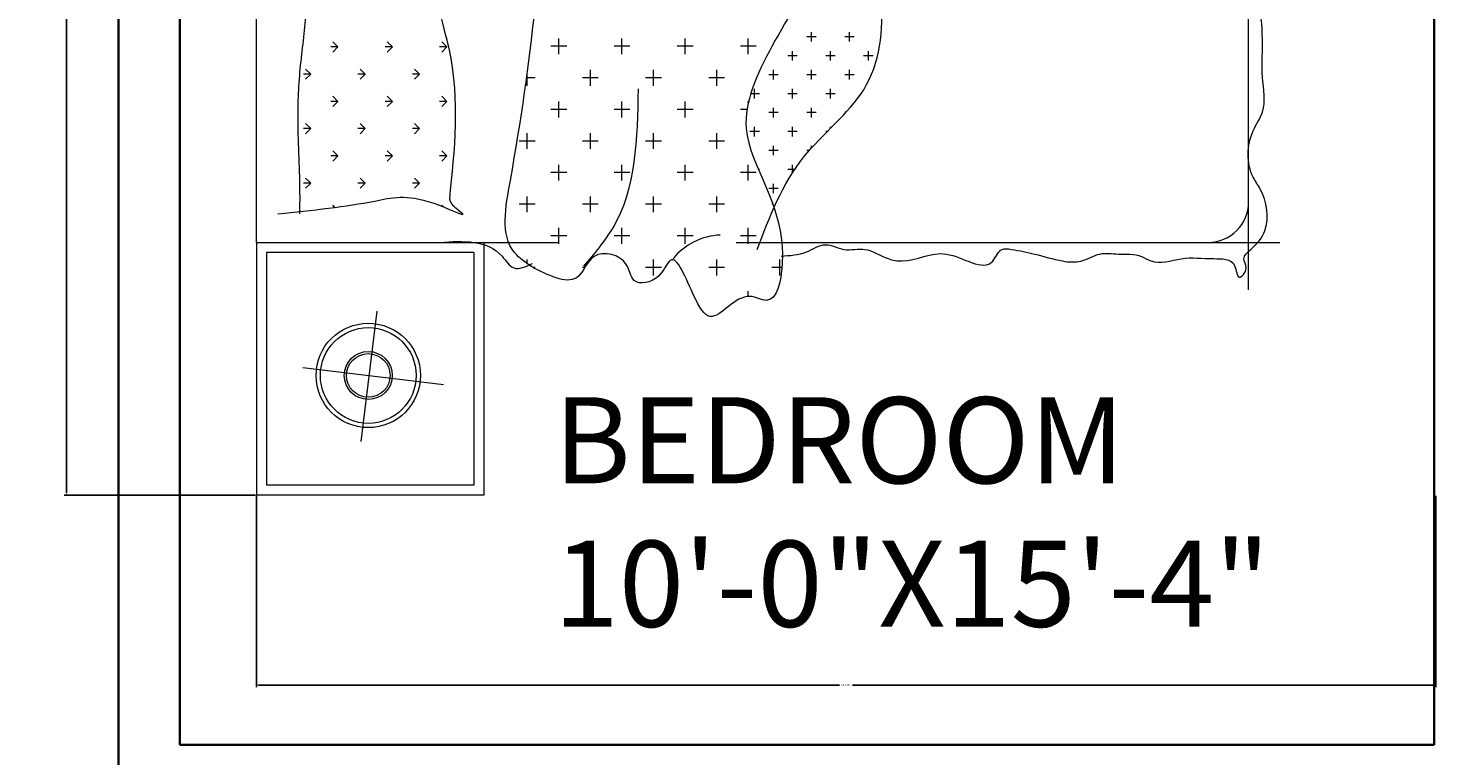
# Model space of a CAD drawing. Units: inches. Extents: x 3731 to 4318, y 1310 to 2388.
# Tile 3 of 57: x 3828 to 3944, y 1393 to 1452. Entities that reach past the tile are written whole.
import ezdxf

# ---------------------------------------------------------------- set-up
doc = ezdxf.new("R2010")
doc.units = ezdxf.units.IN
for name, color, linetype, lineweight in [('A-ANNO-DIMS', 2, 'Continuous', 18), ('A-AREA-IDEN', 7, 'Continuous', 18), ('A-FURN', 8, 'Continuous', 13), ('A-WALL', 7, 'Continuous', 35)]:
    doc.layers.add(name, color=color, linetype=linetype, lineweight=lineweight)
doc.styles.get("Standard").update_dxf_attribs({"font": 'arial.ttf'})
doc.dimstyles.get("Standard").update_dxf_attribs({"dimtxt": 0.18, "dimasz": 0.18, "dimexe": 0.18, "dimexo": 0.0625, "dimgap": 0.09, "dimtad": 0, "dimtih": 1, "dimtoh": 1, "dimdec": 4, "dimzin": 0, "dimdsep": 46, "dimtxsty": 'Standard', "dimcen": 0.09, "dimadec": 0, "dimazin": 0, "dimtfac": 1, "dimtdec": 4, "dimtofl": 0, "dimtmove": 0, "dimatfit": 3, "dimfxl": 1, "dimtolj": 1, "dimtzin": 0, "dimarcsym": 0})

# ---------------------------------------------------------------- blocks, each defined once
blk = doc.blocks.new('A$C200C7901')
for p, q in [((0, 1.8834), (0, 2.3334)), ((0.5, 2.3334), (0, 2.3334)), ((0.5, 2.3334), (0.5, 1.7369)), ((0.5, 2.3334), (0.5, 1.7369)), ((0.5, 2.3334), (2, 2.3334)), ((0.5701, 1.9635), (0.5733, 1.9666)), ((0.5701, 1.9635), (0.5733, 1.9666)), ((0.5, 1.8834), (0, 1.8834)), ((0.4504, 1.782), (0.4504, 1.7863)), ((0.4504, 1.782), (0.4504, 1.7863)), ((0.458, 1.7977), (0.466, 1.7977)), ((0.458, 1.7977), (0.466, 1.7977)), ((0.4504, 1.6834), (0.4504, 1.6883)), ((0.4504, 1.6834), (0.4504, 1.6883)), ((0.4656, 1.6727), (0.466, 1.6727)), ((0.4656, 1.6727), (0.466, 1.6727)), ((0.5597, 1.6727), (0.591, 1.6727)), ((0.5597, 1.6727), (0.591, 1.6727)), ((0.4504, 1.532), (0.4504, 1.5633)), ((0.4347, 1.5477), (0.466, 1.5477)), ((0.6847, 1.5477), (0.716, 1.5477)), ((0.4347, 1.4227), (0.466, 1.4227)), ((0.5, 1.3845), (0.5, 0.3086)), ((0.3931, 1.3602), (0.4035, 1.3602)), ((0.3931, 1.3602), (0.4035, 1.3602)), ((0.4972, 1.3602), (0.5285, 1.3602)), ((0.4972, 1.3602), (0.5285, 1.3602)), ((0.4347, 1.2977), (0.466, 1.2977)), ((0.4347, 1.2977), (0.466, 1.2977)), ((0.4504, 1.2936), (0.4504, 1.3133)), ((0.4504, 1.2936), (0.4504, 1.3133)), ((0.4061, 0.3703), (2.0386, 0.3703))]:
    blk.add_line(p, q)
at = {"linetype": 'ByBlock'}
for p, q in [((0.02, 1.9034), (0.02, 2.3134)), ((0.48, 2.3134), (0.02, 2.3134)), ((0.48, 1.9034), (0.48, 2.3134)), ((0.2524, 2.2412), (0.2186, 1.9635)), ((0.6171, 2.2259), (0.607, 2.236)), ((0.6171, 2.2259), (0.607, 2.236)), ((0.6171, 2.2259), (0.6171, 2.2402)), ((0.6171, 2.2259), (0.6171, 2.2402)), ((0.6171, 2.2259), (0.6272, 2.236)), ((0.6171, 2.2259), (0.6272, 2.236)), ((0.7249, 2.2259), (0.7148, 2.236)), ((0.7249, 2.2259), (0.7148, 2.236)), ((0.7249, 2.2259), (0.7249, 2.2402)), ((0.7249, 2.2259), (0.7249, 2.2402)), ((0.7249, 2.2259), (0.735, 2.236)), ((0.7249, 2.2259), (0.735, 2.236)), ((0.8326, 2.2259), (0.8225, 2.236)), ((0.8326, 2.2259), (0.8225, 2.236)), ((0.8326, 2.2259), (0.8326, 2.2402)), ((0.8326, 2.2259), (0.8326, 2.2402)), ((0.8326, 2.2259), (0.8427, 2.236)), ((0.8326, 2.2259), (0.8427, 2.236)), ((0.5692, 2.178), (0.5733, 2.1822)), ((0.5692, 2.178), (0.5733, 2.1822)), ((0.671, 2.1721), (0.6609, 2.1822)), ((0.671, 2.1721), (0.6609, 2.1822)), ((0.671, 2.172), (0.671, 2.1863)), ((0.671, 2.172), (0.671, 2.1863)), ((0.671, 2.1721), (0.6811, 2.1822)), ((0.671, 2.1721), (0.6811, 2.1822)), ((0.7787, 2.1721), (0.7686, 2.1822)), ((0.7787, 2.1721), (0.7686, 2.1822)), ((0.7787, 2.172), (0.7787, 2.1863)), ((0.7787, 2.172), (0.7787, 2.1863)), ((0.7787, 2.1721), (0.7889, 2.1822)), ((0.7787, 2.1721), (0.7889, 2.1822)), ((0.8865, 2.1721), (0.8764, 2.1822)), ((0.8865, 2.1721), (0.8764, 2.1822)), ((0.8865, 2.172), (0.8865, 2.1863)), ((0.8865, 2.172), (0.8865, 2.1863)), ((0.8865, 2.1721), (0.8966, 2.1822)), ((0.8865, 2.1721), (0.8966, 2.1822)), ((0.3641, 2.0951), (0.1061, 2.1268)), ((0.6171, 2.1182), (0.607, 2.1283)), ((0.6171, 2.1182), (0.607, 2.1283)), ((0.6171, 2.1182), (0.6171, 2.1325)), ((0.6171, 2.1182), (0.6171, 2.1325)), ((0.6171, 2.1182), (0.6272, 2.1283)), ((0.6171, 2.1182), (0.6272, 2.1283)), ((0.7249, 2.1182), (0.7148, 2.1283)), ((0.7249, 2.1182), (0.7148, 2.1283)), ((0.7249, 2.1182), (0.7249, 2.1325)), ((0.7249, 2.1182), (0.7249, 2.1325)), ((0.7249, 2.1182), (0.735, 2.1283)), ((0.7249, 2.1182), (0.735, 2.1283)), ((0.8326, 2.1182), (0.8225, 2.1283)), ((0.8326, 2.1182), (0.8225, 2.1283)), ((0.8326, 2.1182), (0.8326, 2.1325)), ((0.8326, 2.1182), (0.8326, 2.1325)), ((0.8326, 2.1182), (0.8427, 2.1283)), ((0.8326, 2.1182), (0.8427, 2.1283)), ((0.671, 2.0643), (0.6609, 2.0744)), ((0.671, 2.0643), (0.6609, 2.0744)), ((0.671, 2.0643), (0.671, 2.0786)), ((0.671, 2.0643), (0.671, 2.0786)), ((0.671, 2.0643), (0.6811, 2.0744)), ((0.671, 2.0643), (0.6811, 2.0744)), ((0.7787, 2.0643), (0.7686, 2.0744)), ((0.7787, 2.0643), (0.7686, 2.0744)), ((0.7787, 2.0643), (0.7787, 2.0786)), ((0.7787, 2.0643), (0.7787, 2.0786)), ((0.7787, 2.0643), (0.7889, 2.0744)), ((0.7787, 2.0643), (0.7889, 2.0744)), ((0.8865, 2.0643), (0.8764, 2.0744)), ((0.8865, 2.0643), (0.8764, 2.0744)), ((0.8865, 2.0643), (0.8865, 2.0786)), ((0.8865, 2.0643), (0.8865, 2.0786)), ((0.8865, 2.0643), (0.8966, 2.0744)), ((0.8865, 2.0643), (0.8966, 2.0744)), ((0.6171, 2.0104), (0.607, 2.0205)), ((0.6171, 2.0104), (0.607, 2.0205)), ((0.6171, 2.0104), (0.6171, 2.0247)), ((0.6171, 2.0104), (0.6171, 2.0247)), ((0.6171, 2.0104), (0.6272, 2.0205)), ((0.6171, 2.0104), (0.6272, 2.0205)), ((0.7249, 2.0104), (0.7148, 2.0205)), ((0.7249, 2.0104), (0.7148, 2.0205)), ((0.7249, 2.0104), (0.7249, 2.0247)), ((0.7249, 2.0104), (0.7249, 2.0247)), ((0.7249, 2.0104), (0.735, 2.0205)), ((0.7249, 2.0104), (0.735, 2.0205)), ((0.8326, 2.0104), (0.8225, 2.0205)), ((0.8326, 2.0104), (0.8225, 2.0205)), ((0.8326, 2.0104), (0.8326, 2.0247)), ((0.8326, 2.0104), (0.8326, 2.0247)), ((0.8326, 2.0104), (0.8427, 2.0205)), ((0.8326, 2.0104), (0.8427, 2.0205)), ((0.671, 1.9565), (0.6609, 1.9666)), ((0.671, 1.9565), (0.6609, 1.9666)), ((0.671, 1.9565), (0.671, 1.9708)), ((0.671, 1.9565), (0.671, 1.9708)), ((0.671, 1.9565), (0.6811, 1.9666)), ((0.671, 1.9565), (0.6811, 1.9666)), ((0.7787, 1.9565), (0.7686, 1.9666)), ((0.7787, 1.9565), (0.7686, 1.9666)), ((0.7787, 1.9565), (0.7787, 1.9708)), ((0.7787, 1.9565), (0.7787, 1.9708)), ((0.7787, 1.9565), (0.7889, 1.9666)), ((0.7787, 1.9565), (0.7889, 1.9666)), ((0.8865, 1.9565), (0.8764, 1.9666)), ((0.8865, 1.9565), (0.8764, 1.9666)), ((0.8865, 1.9565), (0.8865, 1.9708)), ((0.8865, 1.9565), (0.8865, 1.9708)), ((0.8865, 1.9565), (0.8966, 1.9666)), ((0.8865, 1.9565), (0.8966, 1.9666)), ((0.48, 1.9034), (0.02, 1.9034)), ((0.5754, 1.782), (0.5754, 1.8133)), ((0.5754, 1.782), (0.5754, 1.8133)), ((0.7004, 1.782), (0.7004, 1.8133)), ((0.7004, 1.782), (0.7004, 1.8133)), ((0.5597, 1.7977), (0.591, 1.7977)), ((0.5597, 1.7977), (0.591, 1.7977)), ((0.6847, 1.7977), (0.716, 1.7977)), ((0.6847, 1.7977), (0.716, 1.7977)), ((0.8097, 1.7977), (0.8331, 1.7977)), ((0.8097, 1.7977), (0.8331, 1.7977)), ((0.8254, 1.782), (0.8254, 1.7987)), ((0.8254, 1.782), (0.8254, 1.7987)), ((0.5129, 1.7195), (0.5129, 1.7508)), ((0.5129, 1.7195), (0.5129, 1.7508)), ((0.6379, 1.7195), (0.6379, 1.7508)), ((0.6379, 1.7195), (0.6379, 1.7508)), ((0.7629, 1.7195), (0.7629, 1.7508)), ((0.7629, 1.7195), (0.7629, 1.7508)), ((0.8879, 1.7195), (0.8879, 1.7508)), ((0.8879, 1.7195), (0.8879, 1.7508)), ((0.4972, 1.7352), (0.5285, 1.7352)), ((0.4972, 1.7352), (0.5285, 1.7352)), ((0.6222, 1.7352), (0.6535, 1.7352)), ((0.6222, 1.7352), (0.6535, 1.7352)), ((0.7472, 1.7352), (0.7785, 1.7352)), ((0.7472, 1.7352), (0.7785, 1.7352)), ((0.8722, 1.7352), (0.9035, 1.7352)), ((0.8722, 1.7352), (0.9035, 1.7352)), ((0.5754, 1.657), (0.5754, 1.6883)), ((0.5754, 1.657), (0.5754, 1.6883)), ((0.6847, 1.6727), (0.716, 1.6727)), ((0.6847, 1.6727), (0.716, 1.6727)), ((0.7004, 1.657), (0.7004, 1.6883)), ((0.7004, 1.657), (0.7004, 1.6883)), ((0.8097, 1.6727), (0.841, 1.6727)), ((0.8097, 1.6727), (0.841, 1.6727)), ((0.8254, 1.657), (0.8254, 1.6883)), ((0.8254, 1.657), (0.8254, 1.6883)), ((0.4972, 1.6102), (0.5285, 1.6102)), ((0.4972, 1.6102), (0.5285, 1.6102)), ((0.5129, 1.5945), (0.5129, 1.6258)), ((0.5129, 1.5945), (0.5129, 1.6258)), ((0.6222, 1.6102), (0.6535, 1.6102)), ((0.6222, 1.6102), (0.6535, 1.6102)), ((0.6379, 1.5945), (0.6379, 1.6258)), ((0.6379, 1.5945), (0.6379, 1.6258)), ((0.7472, 1.6102), (0.7785, 1.6102)), ((0.7472, 1.6102), (0.7785, 1.6102)), ((0.7629, 1.5945), (0.7629, 1.6258)), ((0.7629, 1.5945), (0.7629, 1.6258)), ((0.8722, 1.6102), (0.9035, 1.6102)), ((0.8722, 1.6102), (0.9035, 1.6102)), ((0.8879, 1.5945), (0.8879, 1.6258)), ((0.8879, 1.5945), (0.8879, 1.6258)), ((0.4504, 1.532), (0.4504, 1.5633)), ((0.5754, 1.532), (0.5754, 1.5633)), ((0.5754, 1.532), (0.5754, 1.5633)), ((0.7004, 1.532), (0.7004, 1.5633)), ((0.7004, 1.532), (0.7004, 1.5633)), ((0.8254, 1.532), (0.8254, 1.5633)), ((0.8254, 1.532), (0.8254, 1.5633)), ((0.4347, 1.5477), (0.466, 1.5477)), ((0.5597, 1.5477), (0.591, 1.5477)), ((0.5597, 1.5477), (0.591, 1.5477)), ((0.6847, 1.5477), (0.716, 1.5477)), ((0.8097, 1.5477), (0.841, 1.5477)), ((0.8097, 1.5477), (0.841, 1.5477)), ((0.5129, 1.4695), (0.5129, 1.5008)), ((0.5129, 1.4695), (0.5129, 1.5008)), ((0.6379, 1.4695), (0.6379, 1.5008)), ((0.6379, 1.4695), (0.6379, 1.5008)), ((0.7629, 1.4695), (0.7629, 1.5008)), ((0.7629, 1.4695), (0.7629, 1.5008)), ((0.8879, 1.4695), (0.8879, 1.5008)), ((0.8879, 1.4695), (0.8879, 1.5008)), ((0.4972, 1.4852), (0.5285, 1.4852)), ((0.4972, 1.4852), (0.5285, 1.4852)), ((0.6222, 1.4852), (0.6535, 1.4852)), ((0.6222, 1.4852), (0.6535, 1.4852)), ((0.7472, 1.4852), (0.7785, 1.4852)), ((0.7472, 1.4852), (0.7785, 1.4852)), ((0.8722, 1.4852), (0.9035, 1.4852)), ((0.8722, 1.4852), (0.9035, 1.4852)), ((0.4504, 1.407), (0.4504, 1.4383)), ((0.4504, 1.407), (0.4504, 1.4383)), ((0.5754, 1.407), (0.5754, 1.4383)), ((0.5754, 1.407), (0.5754, 1.4383)), ((0.7004, 1.407), (0.7004, 1.4383)), ((0.7004, 1.407), (0.7004, 1.4383)), ((0.8254, 1.407), (0.8254, 1.4383)), ((0.8254, 1.407), (0.8254, 1.4383)), ((0.4347, 1.4227), (0.466, 1.4227)), ((0.5597, 1.4227), (0.591, 1.4227)), ((0.5597, 1.4227), (0.591, 1.4227)), ((0.6847, 1.4227), (0.716, 1.4227)), ((0.6847, 1.4227), (0.716, 1.4227)), ((0.8097, 1.4227), (0.841, 1.4227)), ((0.8097, 1.4227), (0.841, 1.4227)), ((0.5129, 1.3445), (0.5129, 1.3758)), ((0.5129, 1.3445), (0.5129, 1.3758)), ((0.6222, 1.3602), (0.6535, 1.3602)), ((0.6222, 1.3602), (0.6535, 1.3602)), ((0.6379, 1.3445), (0.6379, 1.3758)), ((0.6379, 1.3445), (0.6379, 1.3758)), ((0.7191, 1.3383), (0.7191, 1.357)), ((0.7191, 1.3383), (0.7191, 1.357)), ((0.7629, 1.3627), (0.7629, 1.3758)), ((0.7629, 1.3627), (0.7629, 1.3758)), ((0.7762, 1.3602), (0.7785, 1.3602)), ((0.7762, 1.3602), (0.7785, 1.3602)), ((0.7941, 1.3383), (0.7941, 1.3554)), ((0.7941, 1.3383), (0.7941, 1.3554)), ((0.8722, 1.3602), (0.9035, 1.3602)), ((0.8722, 1.3602), (0.9035, 1.3602)), ((0.8879, 1.3445), (0.8879, 1.3758)), ((0.8879, 1.3445), (0.8879, 1.3758)), ((0.6441, 1.3383), (0.6441, 1.3399)), ((0.6441, 1.3383), (0.6441, 1.3399)), ((0.7097, 1.3477), (0.7285, 1.3477)), ((0.7097, 1.3477), (0.7285, 1.3477)), ((0.7847, 1.3477), (0.8035, 1.3477)), ((0.7847, 1.3477), (0.8035, 1.3477)), ((0.5754, 1.3115), (0.5754, 1.3133)), ((0.5754, 1.3115), (0.5754, 1.3133)), ((0.5972, 1.3102), (0.616, 1.3102)), ((0.5972, 1.3102), (0.616, 1.3102)), ((0.6066, 1.3008), (0.6066, 1.3195)), ((0.6066, 1.3008), (0.6066, 1.3195)), ((0.6722, 1.3102), (0.691, 1.3102)), ((0.6722, 1.3102), (0.691, 1.3102)), ((0.6816, 1.3008), (0.6816, 1.3195)), ((0.6816, 1.3008), (0.6816, 1.3195)), ((0.7472, 1.3102), (0.766, 1.3102)), ((0.7472, 1.3102), (0.766, 1.3102)), ((0.7566, 1.3008), (0.7566, 1.3195)), ((0.7566, 1.3008), (0.7566, 1.3195)), ((0.8222, 1.3102), (0.841, 1.3102)), ((0.8222, 1.3102), (0.841, 1.3102)), ((0.8316, 1.3008), (0.8316, 1.3195)), ((0.8316, 1.3008), (0.8316, 1.3195)), ((0.9066, 1.3008), (0.9066, 1.3028)), ((0.9066, 1.3008), (0.9066, 1.3028)), ((0.6379, 1.2727), (0.6535, 1.2727)), ((0.6379, 1.2727), (0.6535, 1.2727)), ((0.6441, 1.2686), (0.6441, 1.282)), ((0.6441, 1.2686), (0.6441, 1.282)), ((0.7097, 1.2727), (0.7285, 1.2727)), ((0.7097, 1.2727), (0.7285, 1.2727)), ((0.7191, 1.2633), (0.7191, 1.282)), ((0.7191, 1.2633), (0.7191, 1.282)), ((0.7847, 1.2727), (0.8035, 1.2727)), ((0.7847, 1.2727), (0.8035, 1.2727)), ((0.7941, 1.2633), (0.7941, 1.282)), ((0.7941, 1.2633), (0.7941, 1.282)), ((0.8597, 1.2727), (0.8785, 1.2727)), ((0.8597, 1.2727), (0.8785, 1.2727)), ((0.8691, 1.2633), (0.8691, 1.282)), ((0.8691, 1.2633), (0.8691, 1.282)), ((0.6816, 1.2398), (0.6816, 1.2445)), ((0.6816, 1.2398), (0.6816, 1.2445)), ((0.7566, 1.2258), (0.7566, 1.2445)), ((0.7566, 1.2258), (0.7566, 1.2445)), ((0.8316, 1.2258), (0.8316, 1.2445)), ((0.8316, 1.2258), (0.8316, 1.2445)), ((0.9066, 1.2258), (0.9066, 1.2445)), ((0.9066, 1.2258), (0.9066, 1.2445)), ((0.6868, 1.2352), (0.691, 1.2352)), ((0.6868, 1.2352), (0.691, 1.2352)), ((0.7472, 1.2352), (0.766, 1.2352)), ((0.7472, 1.2352), (0.766, 1.2352)), ((0.8222, 1.2352), (0.841, 1.2352)), ((0.8222, 1.2352), (0.841, 1.2352)), ((0.8972, 1.2352), (0.916, 1.2352)), ((0.8972, 1.2352), (0.916, 1.2352)), ((0.7191, 1.2041), (0.7191, 1.207)), ((0.7191, 1.2041), (0.7191, 1.207)), ((0.7255, 1.1977), (0.7285, 1.1977)), ((0.7255, 1.1977), (0.7285, 1.1977)), ((0.7847, 1.1977), (0.8035, 1.1977)), ((0.7847, 1.1977), (0.8035, 1.1977)), ((0.7941, 1.1883), (0.7941, 1.207)), ((0.7941, 1.1883), (0.7941, 1.207)), ((0.8597, 1.1977), (0.8785, 1.1977)), ((0.8597, 1.1977), (0.8785, 1.1977)), ((0.8691, 1.1883), (0.8691, 1.207)), ((0.8691, 1.1883), (0.8691, 1.207)), ((0.7566, 1.1674), (0.7566, 1.1695)), ((0.7566, 1.1674), (0.7566, 1.1695)), ((0.7646, 1.1602), (0.766, 1.1602)), ((0.7646, 1.1602), (0.766, 1.1602)), ((0.8222, 1.1602), (0.841, 1.1602)), ((0.8222, 1.1602), (0.841, 1.1602)), ((0.8316, 1.1508), (0.8316, 1.1695)), ((0.8316, 1.1508), (0.8316, 1.1695)), ((0.8972, 1.1602), (0.916, 1.1602)), ((0.8972, 1.1602), (0.916, 1.1602)), ((0.9066, 1.1508), (0.9066, 1.1695)), ((0.9066, 1.1508), (0.9066, 1.1695)), ((0.8691, 1.1133), (0.8691, 1.132)), ((0.8691, 1.1133), (0.8691, 1.132)), ((0.8597, 1.1227), (0.8785, 1.1227)), ((0.8597, 1.1227), (0.8785, 1.1227))]:
    blk.add_line(p, q, dxfattribs=at)
for radius in [0.1032, 0.0947, 0.0475, 0.0432]:
    blk.add_circle((0.2367, 2.1121), radius, dxfattribs=at)
blk.add_arc((0.3888, 1.4113), 0.1256, 1.9962, 51.1646, dxfattribs=at)
for centre, radius, start, end in [((0.3888, 1.4113), 0.1256, 1.9962, 51.1646), ((0.58, 0.4503), 0.08, 180, 270)]:
    blk.add_arc(centre, radius, start, end)
for points, knots in [([(0.5562, 2.2908), (0.5634, 2.223), (0.5751, 2.1147), (0.6005, 2.0213), (0.5392, 1.8966), (0.5726, 1.9486), (0.5854, 1.951)], [0, 0, 0, 0, 193.119101, 308.278592, 371.468985, 410.593498, 410.593498, 410.593498, 410.593498]), ([(0.5854, 1.951), (0.6835, 1.9407), (0.8425, 1.9242), (1.0374, 2.0054), (1.1564, 1.9255), (1.2274, 1.9841), (1.2052, 2.0751), (1.1815, 2.152), (1.2176, 2.2368), (1.0992, 2.2731), (1.0008, 2.2255), (0.8698, 2.246), (0.7481, 2.2548), (0.6426, 2.2473), (0.5746, 2.2478), (0.5562, 2.2479)], [0, 0, 0, 0, 292.165466, 473.33038, 601.631673, 630.723769, 727.138505, 836.819956, 887.958136, 954.42438, 1118.989809, 1227.016542, 1338.750986, 1487.447361, 1542.751028, 1542.751028, 1542.751028, 1542.751028]), ([(0.4485, 1.7835), (0.4321, 1.7496), (0.4062, 1.6964), (0.49, 1.6713), (0.4719, 1.5969), (0.4123, 1.592), (0.4233, 1.5337), (0.4954, 1.5086), (0.4012, 1.4738), (0.3253, 1.4306), (0.4113, 1.3764), (0.3688, 1.3065), (0.5579, 1.2663), (0.741, 1.4533), (1.1127, 1.1109), (1.4811, 1.2478), (1.7885, 1.3492), (2.0357, 1.1637), (2.0748, 1.2974), (2.0876, 1.349), (2.0192, 1.3805), (2.0564, 1.4298), (2.0588, 1.4846), (1.9759, 1.5349), (2.1004, 1.5845), (2.0397, 1.6519), (1.971, 1.7053), (2.1104, 1.8981), (1.5946, 1.7967), (1.2448, 1.7472), (0.8129, 1.7935), (0.4953, 1.8548), (0.4582, 1.7983), (0.4485, 1.7835)], [0, 0, 0, 0, 88.420092, 139.08588, 204.302936, 239.695496, 287.801042, 327.365471, 412.960499, 463.626286, 552.059846, 584.668336, 662.614915, 940.993281, 1309.926334, 1844.022653, 1996.276242, 2316.43048, 2341.441004, 2404.707416, 2449.463774, 2514.680778, 2538.40571, 2613.031547, 2697.13096, 2760.903931, 2822.692699, 2945.47, 3215.060018, 3725.584917, 4361.974444, 4504.671998, 4555.32777, 4555.32777, 4555.32777, 4555.32777]), ([(0.4856, 1.3429), (0.5504, 1.3182), (0.6715, 1.2721), (0.8374, 1.0498), (1.1164, 1.1183), (1.3878, 1.1816), (1.5888, 1.1102), (1.8403, 1.1127), (1.9415, 1.2178), (2.0032, 1.2819)], [0, 0, 0, 0, 205.411753, 383.654933, 772.067458, 921.644661, 1226.793228, 1388.983508, 1642.292305, 1642.292305, 1642.292305, 1642.292305])]:
    blk.add_open_spline(points, degree=3, knots=knots)
for points, knots in [([(0.5, 1.9703), (0.5029, 1.9235), (0.5066, 1.8648), (0.4398, 1.8252), (0.452, 1.8005), (0.4585, 1.7872)], [0, 0, 0, 0, 126.315232, 158.854004, 196.789047, 196.789047, 196.789047, 196.789047]), ([(0.5, 1.9703), (0.5029, 1.9235), (0.5066, 1.8648), (0.4398, 1.8252), (0.452, 1.8005), (0.4585, 1.7872)], [0, 0, 0, 0, 126.315232, 158.854004, 196.789047, 196.789047, 196.789047, 196.789047]), ([(0.4532, 1.6853), (0.4776, 1.6644), (0.574, 1.582), (0.7055, 1.5794), (0.8037, 1.5774)], [0, 0, 0, 0, 94.920667, 374.457292, 374.457292, 374.457292, 374.457292]), ([(0.4532, 1.6853), (0.4776, 1.6644), (0.574, 1.582), (0.7055, 1.5794), (0.8037, 1.5774)], [0, 0, 0, 0, 94.920667, 374.457292, 374.457292, 374.457292, 374.457292]), ([(0.473, 1.2954), (0.4739, 1.2781), (0.4755, 1.2477), (0.5032, 1.2084), (0.4801, 1.1701), (0.4928, 1.1255), (0.4674, 1.0912), (0.4579, 1.0351), (0.501, 0.9724), (0.4311, 0.8832), (0.4902, 0.8637), (0.4843, 0.8288), (0.4774, 0.7906), (0.4625, 0.7457), (0.459, 0.6999), (0.4816, 0.6664), (0.4748, 0.625), (0.4791, 0.5889), (0.4533, 0.5528), (0.4738, 0.5004), (0.4658, 0.4502), (0.4696, 0.3946), (0.4189, 0.3935), (0.4493, 0.3684), (0.4694, 0.3857), (0.4922, 0.3576), (0.5297, 0.3262), (0.5917, 0.3353), (0.6454, 0.3754), (0.7083, 0.3741), (0.7643, 0.3328), (0.826, 0.346), (0.925, 0.3388), (1.0353, 0.3593), (1.1561, 0.3744), (1.2477, 0.3154), (1.3302, 0.3474), (1.4086, 0.3512), (1.5217, 0.3878), (1.6362, 0.3176), (1.7682, 0.3285), (1.8402, 0.3019), (1.9071, 0.3529), (1.9647, 0.3412), (2.0795, 0.2948), (2.0472, 0.3498), (2.0343, 0.3772), (2.0435, 0.43), (2.0109, 0.5782), (2.0746, 0.4643), (2.0805, 0.584), (2.0084, 0.5979), (2.0343, 0.6846), (2.0344, 0.746), (2.0293, 0.8096), (2.0489, 0.8545), (2.0652, 0.9218), (1.9842, 0.9297), (2.0007, 1.0162), (2.0367, 1.0585), (2.0367, 1.1102), (2.0457, 1.1647), (2.0226, 1.2084), (2.0234, 1.2306), (2.0236, 1.2352)], [0, 0, 0, 0, 51.660678, 90.967412, 128.902454, 170.303599, 219.852997, 247.834962, 336.321557, 429.35469, 458.821847, 477.222321, 524.135809, 581.038434, 617.839381, 657.146115, 693.947125, 740.178081, 760.753248, 820.731705, 885.133458, 928.777044, 953.563729, 976.574207, 995.553042, 1018.563482, 1064.584401, 1147.951297, 1174.787598, 1266.851571, 1308.018447, 1377.066427, 1441.511314, 1608.245014, 1714.11869, 1792.771707, 1913.247991, 1954.931389, 2029.864445, 2259.189419, 2305.221512, 2429.507982, 2456.344283, 2543.92595, 2627.925037, 2662.96218, 2687.736879, 2719.937755, 2839.540991, 2875.47895, 2953.681041, 2993.270313, 3066.872333, 3154.395764, 3200.397042, 3248.426375, 3312.828127, 3347.881398, 3444.484026, 3481.577522, 3518.665244, 3592.267265, 3644.719162, 3658.519501, 3658.519501, 3658.519501, 3658.519501])]:
    blk.add_open_spline(points, degree=3, knots=knots, dxfattribs=at)
blk = doc.blocks.new('*D16')
at = {"layer": 'A-ANNO-DIMS', "color": 0, "lineweight": -2, "transparency": 16777216}
for p, q in [((3846.36, 1516.63), (3830.8, 1516.63)), ((3830.98, 1516.45), (3830.98, 1465.34)), ((3830.98, 1413.86), (3830.98, 1464.97)), ((3846.36, 1413.68), (3830.8, 1413.68))]:
    blk.add_line(p, q, dxfattribs=at)
at = {"layer": 'A-ANNO-DIMS', "color": 0, "transparency": 16777216}
for points in [[(3830.95, 1516.45), (3831.01, 1516.45), (3830.98, 1516.63)], [(3830.95, 1413.86), (3831.01, 1413.86), (3830.98, 1413.68)]]:
    blk.add_solid(points, dxfattribs=at)
at = {"layer": 'Defpoints', "color": 0, "transparency": 16777216}
for p in [(3830.98, 1516.63), (3846.43, 1516.63), (3846.43, 1413.68)]:
    blk.add_point(p, dxfattribs=at)
at = {"layer": 'A-ANNO-DIMS', "color": 0, "transparency": 16777216, "insert": (3830.98, 1465.15), "char_height": 0.18, "attachment_point": 5}
blk.add_mtext('\\A1;BED SET 103 TYP.', dxfattribs=at)
blk = doc.blocks.new('*D17')
at = {"layer": 'A-ANNO-DIMS', "color": 0, "lineweight": -2, "transparency": 16777216}
for p, q in [((3846.43, 1413.62), (3846.43, 1398.06)), ((3942.35, 1413.62), (3942.35, 1398.06)), ((3846.61, 1398.24), (3893.86, 1398.24)), ((3942.17, 1398.24), (3894.91, 1398.24))]:
    blk.add_line(p, q, dxfattribs=at)
at = {"layer": 'A-ANNO-DIMS', "color": 0, "transparency": 16777216}
for points in [[(3846.61, 1398.27), (3846.61, 1398.21), (3846.43, 1398.24)], [(3942.17, 1398.27), (3942.17, 1398.21), (3942.35, 1398.24)]]:
    blk.add_solid(points, dxfattribs=at)
at = {"layer": 'Defpoints', "color": 0, "transparency": 16777216}
for p in [(3846.43, 1413.68), (3942.35, 1413.68), (3846.43, 1398.24)]:
    blk.add_point(p, dxfattribs=at)
at = {"layer": 'A-ANNO-DIMS', "color": 0, "transparency": 16777216, "insert": (3894.39, 1398.24), "char_height": 0.18, "attachment_point": 5}
blk.add_mtext('\\A1;96 TYP.', dxfattribs=at)
blk = doc.blocks.new('*D32')
at = {"layer": 'A-ANNO-DIMS', "color": 0, "lineweight": -2, "transparency": 16777216}
for p, q in [((4269.21, 1592.32), (4269.21, 1310.25)), ((3835.21, 1359.32), (3835.21, 1310.25)), ((3835.39, 1310.43), (4051.92, 1310.43)), ((4269.03, 1310.43), (4052.5, 1310.43))]:
    blk.add_line(p, q, dxfattribs=at)
at = {"layer": 'A-ANNO-DIMS', "color": 0, "transparency": 16777216}
for points in [[(3835.39, 1310.46), (3835.39, 1310.4), (3835.21, 1310.43)], [(4269.03, 1310.46), (4269.03, 1310.4), (4269.21, 1310.43)]]:
    blk.add_solid(points, dxfattribs=at)
at = {"layer": 'Defpoints', "color": 0, "transparency": 16777216}
for p in [(4269.21, 1592.38), (3835.21, 1359.38), (4269.21, 1310.43)]:
    blk.add_point(p, dxfattribs=at)
at = {"layer": 'A-ANNO-DIMS', "color": 0, "transparency": 16777216, "insert": (4052.21, 1310.43), "char_height": 0.18, "attachment_point": 5}
blk.add_mtext('\\A1;434', dxfattribs=at)
blk = doc.blocks.new('*D33')
at = {"layer": 'A-ANNO-DIMS', "color": 0, "lineweight": -2, "transparency": 16777216}
for p, q in [((3835.15, 2338.38), (3731.41, 2338.38)), ((3731.59, 2338.2), (3731.59, 1849.06)), ((3731.59, 1359.56), (3731.59, 1848.7)), ((3835.15, 1359.38), (3731.41, 1359.38))]:
    blk.add_line(p, q, dxfattribs=at)
at = {"layer": 'A-ANNO-DIMS', "color": 0, "transparency": 16777216}
for points in [[(3731.56, 2338.2), (3731.62, 2338.2), (3731.59, 2338.38)], [(3731.56, 1359.56), (3731.62, 1359.56), (3731.59, 1359.38)]]:
    blk.add_solid(points, dxfattribs=at)
at = {"layer": 'Defpoints', "color": 0, "transparency": 16777216}
for p in [(3731.59, 2338.38), (3835.21, 2338.38), (3835.21, 1359.38)]:
    blk.add_point(p, dxfattribs=at)
at = {"layer": 'A-ANNO-DIMS', "color": 0, "transparency": 16777216, "insert": (3731.59, 1848.88), "char_height": 0.18, "attachment_point": 5}
blk.add_mtext('\\A1;979', dxfattribs=at)

msp = doc.modelspace()

# ---------------------------------------------------------------- linework, layer by layer
at = {"layer": 'A-WALL'}
for p, q in [((3835.21, 2338.38), (3835.21, 1359.38)), ((3840.21, 1549.38), (3840.21, 1393.38)), ((3942.21, 1489.38), (3942.21, 1393.38)), ((3840.21, 1393.38), (3942.21, 1393.38))]:
    msp.add_line(p, q, dxfattribs=at)

# ---------------------------------------------------------------- block references
at = {"layer": 'A-FURN', "xscale": 41.1071563136412, "yscale": 41.1071563136412, "zscale": 41.1071563136412, "rotation": 90}
msp.add_blockref('A$C200C7901', (3942.35, 1413.68), dxfattribs=at)

# ---------------------------------------------------------------- texts
at = {"layer": 'A-AREA-IDEN', "insert": (3870.61, 1421.64), "char_height": 7, "attachment_point": 1}
msp.add_mtext_dynamic_manual_height_columns('BEDROOM\\P10\'-0"X15\'-4"', width=47.0437, gutter_width=12.5, heights=[0], dxfattribs=at)

# ---------------------------------------------------------------- dimensions: what is measured, and where the dimension line sits
at = {"layer": 'A-ANNO-DIMS'}
dim = msp.add_linear_dim(base=(3731.59, 2338.38), p1=(3835.21, 1359.38), p2=(3835.21, 2338.38), angle=90, dimstyle='Standard', override={"dimdec": 0, "dimlfac": 1, "dimrnd": 0, "dimzin": 0, "dimdsep": 46, "dimlunit": 2}, dxfattribs=at)
dim.commit()
dim.dimension.update_dxf_attribs({"geometry": '*D33', "text_midpoint": (3731.59, 1848.88)})
dim = msp.add_linear_dim(base=(4269.21, 1310.43), p1=(3835.21, 1359.38), p2=(4269.21, 1592.38), dimstyle='Standard', override={"dimdec": 0, "dimlfac": 1, "dimrnd": 0, "dimzin": 0, "dimdsep": 46, "dimlunit": 2}, dxfattribs=at)
dim.commit()
dim.dimension.update_dxf_attribs({"geometry": '*D32', "text_midpoint": (4052.21, 1310.43)})
for base, p1, p2, angle, text, picture, middle in [((3830.98, 1516.63), (3846.43, 1413.68), (3846.43, 1516.63), 90, 'BED SET <> TYP.', '*D16', (3830.98, 1465.15)), ((3846.43, 1398.24), (3942.35, 1413.68), (3846.43, 1413.68), 180, '<> TYP.', '*D17', (3894.39, 1398.24))]:
    dim = msp.add_linear_dim(base=base, p1=p1, p2=p2, angle=angle, text=text, dimstyle='Standard', override={"dimdec": 0, "dimlfac": 1, "dimrnd": 0, "dimzin": 0, "dimdsep": 46, "dimlunit": 2}, dxfattribs=at)
    dim.commit()
    dim.dimension.update_dxf_attribs({"geometry": picture, "text_midpoint": middle})

doc.saveas('drawing.dxf')
